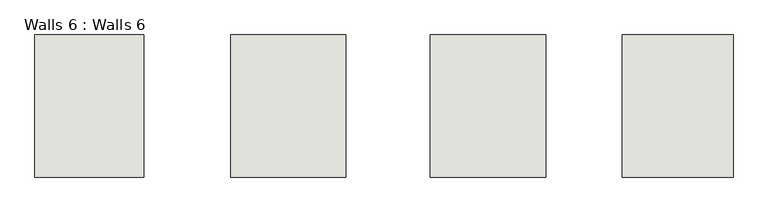
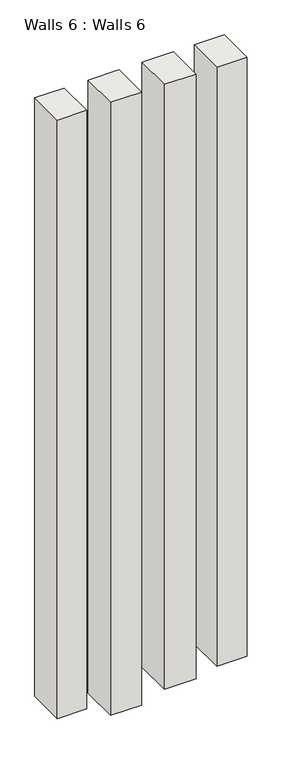
"""IFC4 building model written with IfcOpenShell, lengths in millimetres: wall geometry, Walls 6 : Walls 6."""

from ifc_helpers import new_model, si_unit, frame, origin, place, context, project, spatial, polyline, outline, extrude, source, transform, mapped, element, save


def walls_6_walls_6_eb98cddc(model_context):
    return source(origin(), model_context, "Body", "SweptSolid", [
        extrude(outline(polyline([(-8298.5172806, -2688.1885822), (-8530.7557758, -2688.1885822), (-8530.7557758, -2383.3885822), (-8298.5172806, -2383.3885822), (-8298.5172806, -2688.1885822)])), frame((0.0, 0.0, 7219.3838479), z_axis=(0.0, 0.0, 1.0), x_axis=(1.0, 0.0, 0.0)), (0.0, 0.0, 1.0), 4972.6161521),
        extrude(outline(polyline([(-7866.5398384, -2688.1885822), (-8112.268695, -2688.1885822), (-8112.268695, -2383.3885822), (-7866.5398384, -2383.3885822), (-7866.5398384, -2688.1885822)])), frame((0.0, 0.0, 7099.5980522), z_axis=(0.0, 0.0, 1.0), x_axis=(1.0, 0.0, 0.0)), (0.0, 0.0, 1.0), 5092.4019478),
        extrude(outline(polyline([(-7438.5557758, -2688.1885822), (-7685.9461253, -2688.1885822), (-7685.9461253, -2383.3885822), (-7438.5557758, -2383.3885822), (-7438.5557758, -2688.1885822)])), frame((0.0, 0.0, 7167.9637665), z_axis=(0.0, 0.0, 1.0), x_axis=(1.0, 0.0, 0.0)), (0.0, 0.0, 1.0), 5024.0362335),
        extrude(outline(polyline([(-7038.2481941, -2688.1885822), (-7275.704932, -2688.1885822), (-7275.704932, -2383.3885822), (-7038.2481941, -2383.3885822), (-7038.2481941, -2688.1885822)])), frame((0.0, 0.0, 7214.7134922), z_axis=(0.0, 0.0, 1.0), x_axis=(1.0, 0.0, 0.0)), (0.0, 0.0, 1.0), 4977.2865078),
    ])


if __name__ == "__main__":
    model = new_model("IFC4")
    model_context = context("Model", 3, world=origin())
    ifc_project = project(units=[si_unit("LENGTHUNIT", "METRE", prefix="MILLI")], contexts=[model_context])
    site = spatial("IfcSite", under=ifc_project)
    building = spatial("IfcBuilding", under=site)
    placement = place(None, origin())
    walls_6_walls_6_shape = walls_6_walls_6_eb98cddc(model_context)
    element("IfcWall", 1, ObjectType="Walls 6 : Walls 6", at=placement, inside=building, context=model_context, shape_type="MappedRepresentation", body=[
        mapped(walls_6_walls_6_shape, transform((0.0, 0.0, 0.0), x_axis=(1.0, 0.0, 0.0), y_axis=(0.0, 1.0, 0.0), z_axis=(0.0, 0.0, 1.0))),
    ])
    save(model, "model.ifc")

# Revit data of these elements
# Element 1 (IfcWall, "Walls 6 : Walls 6")
#   Materials on its faces: "Default Wall"
# Materials
#   "Default Wall": colour RGB 128 128 128, transparency 0
